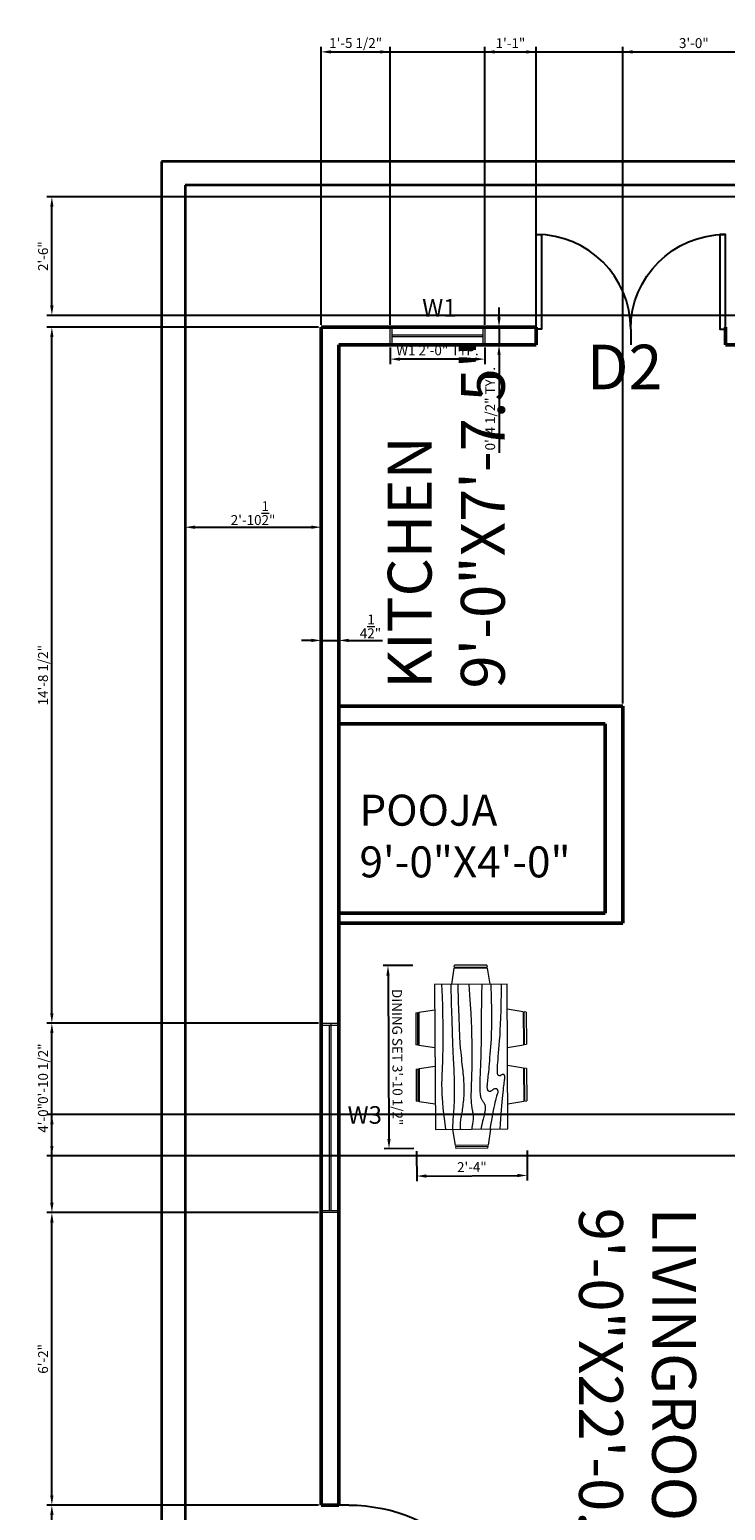
# Model space of a CAD drawing. Units: inches. Extents: x 2727 to 5054, y 1285 to 3233.
# Tile 2 of 3: x 2727 to 2903, y 1525 to 1900. Entities that reach past the tile are written whole.
import ezdxf

# ---------------------------------------------------------------- set-up
doc = ezdxf.new("R2010")
doc.units = ezdxf.units.IN
for name, color, linetype, lineweight in [('A-ANNO-TEXT', 1, 'Continuous', 18), ('A-AREA-IDEN', 1, 'Continuous', 18), ('A-WALL-SITE', 7, 'Continuous', 35), ('DIMENSIONS', 9, 'Continuous', 18), ('doors', 5, 'Continuous', 25), ('furniture', 8, 'Continuous', 18), ('walls', 7, 'Continuous', 50), ('windows', 3, 'Continuous', 18)]:
    doc.layers.add(name, color=color, linetype=linetype, lineweight=lineweight)
doc.styles.get("Standard").update_dxf_attribs({"font": 'arial.ttf'})
doc.dimstyles.new('ISO-25', dxfattribs={"dimtxt": 2.5, "dimasz": 2.5, "dimexe": 1.25, "dimexo": 0.625, "dimtad": 1, "dimlunit": 4, "dimtxsty": 'Standard', "dimcen": 2.5, "dimadec": 0, "dimazin": 0, "dimtfac": 1, "dimtmove": 0, "dimatfit": 3, "dimfxl": 1, "dimarcsym": 0})

# ---------------------------------------------------------------- blocks, each defined once
blk = doc.blocks.new('*U2')
for p, q in [((0, 0), (0, -5)), ((30, 0), (30, -5))]:
    blk.add_line(p, q)
blk.add_lwpolyline([(0, 0), (0, 30), (1.75, 30), (1.75, 0)], close=True)
blk.add_arc((0, 0), 30, 0, 90)
blk = doc.blocks.new('Dining Set - 36 x 72 in.')
for p, q in [((-22.2343, 26.00059), (-23.4847, 17.99762)), ((-22.2304, 26), (-5.7608, 26)), ((-22, 27.5), (-22.1562, 26.50042)), ((-5.8416, 26.5), (-22.1534, 26.5)), ((-22, 27.5), (-6, 27.5)), ((-5.8437, 26.49966), (-6, 27.5)), ((-4.5152, 17.99762), (-5.7655, 25.99926)), ((5.7657, 26.00059), (4.5153, 17.99762)), ((5.7696, 26), (22.2392, 26)), ((6, 27.5), (5.8438, 26.50042)), ((22.1584, 26.5), (5.8466, 26.5)), ((6, 27.5), (22, 27.5)), ((22.1563, 26.49966), (22, 27.5)), ((23.4848, 17.99762), (22.2345, 25.99926)), ((36, 18), (-36, 18)), ((-36, 18), (-36, -18)), ((36, -18), (36, 18)), ((-45.5, 8), (-44.5004, 8.15617)), ((-45.5, 8), (-45.5, -8)), ((-44.5, -8.15843), (-44.5, 8.15338)), ((-44.0006, 8.23428), (-35.9976, 9.48474)), ((-44, 8.23041), (-44, -8.23915)), ((44.0006, 8.23428), (35.9976, 9.48474)), ((44, 8.23041), (44, -8.23915)), ((44.5, -8.15843), (44.5, 8.15338)), ((45.5, 8), (44.5005, 8.15617)), ((45.5, 8), (45.5, -8)), ((-44.4997, -8.15631), (-45.5, -8)), ((-35.9976, -9.48476), (-43.9993, -8.2345)), ((35.9976, -9.48476), (43.9993, -8.2345)), ((44.4997, -8.15631), (45.5, -8)), ((-36, -18), (36, -18)), ((-22.2343, -26.0006), (-23.4847, -17.99762)), ((-4.5152, -17.99762), (-5.7655, -25.99928)), ((5.7657, -26.0006), (4.5153, -17.99762)), ((23.4848, -17.99762), (22.2345, -25.99928)), ((-22.2304, -26), (-5.7608, -26)), ((-22, -27.5), (-22.1562, -26.50044)), ((-5.8416, -26.5), (-22.1534, -26.5)), ((-22, -27.5), (-6, -27.5)), ((-5.8437, -26.49967), (-6, -27.5)), ((5.7696, -26), (22.2392, -26)), ((6, -27.5), (5.8438, -26.50044)), ((22.1584, -26.5), (5.8466, -26.5)), ((6, -27.5), (22, -27.5)), ((22.1563, -26.49967), (22, -27.5))]:
    blk.add_line(p, q)
for points in [[(-36, 15), (-31.1772, 14.97754), (-26.8079, 14.91406), (-22.8538, 14.81543), (-19.276, 14.6875), (-16.0362, 14.53613), (-13.0957, 14.36718), (-10.4159, 14.18652), (-7.9583, 14), (-5.6904, 13.81315), (-3.6035, 13.63021), (-1.6954, 13.45508), (0.0365, 13.29166), (1.5945, 13.14388), (2.9811, 13.01562), (4.1988, 12.9108), (5.25, 12.83333), (6.1393, 12.78613), (6.8802, 12.76823), (7.4883, 12.77767), (7.9792, 12.8125), (8.3685, 12.87077), (8.6719, 12.95052), (8.9049, 13.0498), (9.0833, 13.16666), (9.2205, 13.29899), (9.3216, 13.44401), (9.3895, 13.59879), (9.4271, 13.76041), (9.4373, 13.92594), (9.4232, 14.09245), (9.3875, 14.257), (9.3333, 14.41666), (9.2638, 14.56917), (9.1836, 14.71484), (9.0975, 14.85465), (9.0104, 14.98958), (8.9272, 15.1206), (8.8529, 15.2487), (8.7922, 15.37483), (8.75, 15.5), (8.7305, 15.62467), (8.7344, 15.74739), (8.7617, 15.86621), (8.8125, 15.97916), (8.8867, 16.08431), (8.9844, 16.17968), (9.1055, 16.26334), (9.25, 16.33333), (9.4189, 16.38802), (9.6172, 16.42708), (9.8506, 16.45052), (10.125, 16.45833), (10.4463, 16.45052), (10.8203, 16.42708), (11.2529, 16.38802), (11.75, 16.33333), (12.3184, 16.26318), (12.9694, 16.17838), (13.7151, 16.07991), (14.5677, 15.96875), (15.5395, 15.84586), (16.6426, 15.71224), (17.8893, 15.56884), (19.2917, 15.41666), (20.859, 15.25667), (22.5879, 15.08984), (24.4721, 14.91715), (26.5052, 14.73958), (28.6809, 14.5581), (30.9929, 14.3737), (33.4347, 14.18733), (36, 14)], [(-36, 10), (-28.9766, 10.14274), (-23.1725, 10.20442), (-18.4241, 10.19775), (-14.5677, 10.13541), (-11.4399, 10.03011), (-8.877, 9.89453), (-6.7154, 9.74137), (-4.7917, 9.58333), (-2.9698, 9.43082), (-1.2246, 9.28515), (0.4415, 9.14534), (2.026, 9.01041), (3.5266, 8.87939), (4.9408, 8.7513), (6.266, 8.62516), (7.5, 8.5), (8.6411, 8.37549), (9.6914, 8.2539), (10.6538, 8.13818), (11.5312, 8.03125), (12.3267, 7.93603), (13.043, 7.85547), (13.6831, 7.79248), (14.25, 7.75), (14.7471, 7.7303), (15.1797, 7.73307), (15.5537, 7.75732), (15.875, 7.80208), (16.1494, 7.86637), (16.3828, 7.94922), (16.5811, 8.04964), (16.75, 8.16666), (16.8944, 8.29915), (17.0143, 8.44531), (17.1089, 8.60319), (17.1771, 8.77083), (17.218, 8.94629), (17.2305, 9.1276), (17.2137, 9.31282), (17.1667, 9.5), (17.0895, 9.6875), (16.987, 9.875), (16.8649, 10.0625), (16.7292, 10.25), (16.5856, 10.4375), (16.4401, 10.625), (16.2985, 10.8125), (16.1667, 11), (16.05, 11.18733), (15.9518, 11.3737), (15.8752, 11.5581), (15.8229, 11.73958), (15.798, 11.91715), (15.8034, 12.08984), (15.842, 12.25667), (15.9167, 12.41666), (16.0295, 12.56836), (16.1784, 12.70833), (16.3605, 12.83268), (16.5729, 12.9375), (16.8127, 13.01888), (17.0768, 13.07291), (17.3625, 13.0957), (17.6667, 13.08333), (17.9894, 13.03312), (18.3418, 12.94726), (18.7382, 12.82918), (19.1927, 12.68229), (19.7195, 12.51001), (20.3327, 12.31575), (21.0465, 12.10294), (21.875, 11.875), (22.8357, 11.63354), (23.959, 11.37304), (25.2786, 11.08618), (26.8282, 10.76562), (28.6414, 10.40405), (30.752, 9.99414), (33.1936, 9.52856), (36, 9)], [(-36, 5.5), (-30.7157, 5.3348), (-26.069, 5.20963), (-21.9946, 5.11767), (-18.4271, 5.05208), (-15.3009, 5.00602), (-12.5508, 4.97265), (-10.1112, 4.94515), (-7.9167, 4.91666), (-5.909, 4.88167), (-4.0586, 4.83984), (-2.3429, 4.79215), (-0.7396, 4.73958), (0.7739, 4.6831), (2.22, 4.6237), (3.6213, 4.56233), (5, 4.5), (6.373, 4.43782), (7.7344, 4.3776), (9.0723, 4.32129), (10.375, 4.27083), (11.6309, 4.22819), (12.8281, 4.19531), (13.9551, 4.17415), (15, 4.16666), (15.954, 4.17448), (16.819, 4.19791), (17.6001, 4.23698), (18.3021, 4.29166), (18.9299, 4.36198), (19.4883, 4.44791), (19.9823, 4.54948), (20.4167, 4.66666), (20.7969, 4.79899), (21.1302, 4.94401), (21.4245, 5.09879), (21.6875, 5.26041), (21.9271, 5.42594), (22.1511, 5.59245), (22.3672, 5.757), (22.5834, 5.91666), (22.8065, 6.06868), (23.0404, 6.21093), (23.2879, 6.34147), (23.5521, 6.45833), (23.8358, 6.55957), (24.142, 6.64323), (24.4735, 6.70735), (24.8334, 6.75), (25.2235, 6.76969), (25.642, 6.76692), (26.0858, 6.74267), (26.5521, 6.69791), (27.0379, 6.63362), (27.5404, 6.55078), (28.0565, 6.45036), (28.5834, 6.33333), (29.1242, 6.19987), (29.7071, 6.04687), (30.3661, 5.87044), (31.1354, 5.66666), (32.0493, 5.43164), (33.142, 5.16146), (34.4475, 4.85221), (36, 4.5)], [(-36, -1), (-30.7915, -0.6591), (-26.0195, -0.38216), (-21.6519, -0.16284), (-17.6563, 0.00521), (-14.0005, 0.12833), (-10.6523, 0.21289), (-7.5796, 0.26522), (-4.75, 0.29166), (-2.134, 0.29793), (0.2878, 0.28711), (2.5317, 0.26163), (4.6146, 0.22396), (6.5529, 0.17651), (8.3633, 0.12174), (10.0623, 0.06209), (11.6667, 0), (13.1899, -0.06201), (14.6341, -0.1211), (15.9982, -0.17432), (17.2813, -0.21875), (18.4823, -0.25147), (19.6003, -0.26953), (20.6343, -0.27002), (21.5834, -0.25), (22.4481, -0.20768), (23.2357, -0.14584), (23.9549, -0.06836), (24.6146, 0.02083), (25.2235, 0.11784), (25.7904, 0.21875), (26.3241, 0.31966), (26.8334, 0.41666), (27.3265, 0.50618), (27.8099, 0.58593), (28.2894, 0.65397), (28.7709, 0.70833), (29.2601, 0.74707), (29.763, 0.76823), (30.2855, 0.76985), (30.8334, 0.75), (31.4088, 0.70784), (31.9994, 0.64713), (32.589, 0.57275), (33.1615, 0.48958), (33.7008, 0.4025), (34.1908, 0.3164), (34.6153, 0.23616), (34.9584, 0.16666), (35.2099, 0.11165), (35.3848, 0.07031), (35.504, 0.04069), (35.5886, 0.02083), (35.6594, 0.00879), (35.7377, 0.0026), (35.8442, 0.00032), (36, 0)], [(-36, -6.5), (-27.1843, -6.31267), (-20.084, -6.1263), (-14.469, -5.9419), (-10.1094, -5.76042), (-6.7752, -5.58285), (-4.2363, -5.41016), (-2.2629, -5.24333), (-0.625, -5.08334), (0.8708, -4.93099), (2.2715, -4.78646), (3.5872, -4.64974), (4.8281, -4.52084), (6.0046, -4.39974), (7.127, -4.28646), (8.2053, -4.18099), (9.25, -4.08334), (10.2705, -3.99382), (11.2734, -3.91407), (12.2647, -3.84603), (13.25, -3.79167), (14.2354, -3.75293), (15.2266, -3.73177), (16.2295, -3.73015), (17.25, -3.75), (18.2912, -3.79248), (19.3451, -3.85547), (20.4009, -3.93604), (21.4479, -4.03125), (22.4754, -4.13819), (23.4727, -4.25391), (24.4289, -4.37549), (25.3334, -4.5), (26.1785, -4.62492), (26.9694, -4.74935), (27.7145, -4.87281), (28.4219, -4.99479), (29.1, -5.11483), (29.7572, -5.23242), (30.4016, -5.34709), (31.0417, -5.45834), (31.6837, -5.56437), (32.3262, -5.65821), (32.9658, -5.73153), (33.599, -5.77604), (34.2224, -5.78345), (34.8327, -5.74545), (35.4264, -5.65373), (36, -5.5)], [(-36, -10), (-26.4022, -9.81299), (-18.4675, -9.62891), (-11.9839, -9.45069), (-6.7396, -9.28125), (-2.5226, -9.12354), (0.8789, -8.98047), (3.6769, -8.85498), (6.0833, -8.75), (8.2767, -8.66765), (10.3021, -8.60677), (12.1712, -8.56543), (13.8958, -8.54167), (15.4876, -8.53353), (16.9583, -8.53907), (18.3197, -8.55632), (19.5834, -8.58334), (20.7616, -8.61841), (21.8685, -8.66081), (22.9188, -8.71004), (23.9271, -8.76563), (24.9081, -8.82707), (25.8763, -8.89388), (26.8465, -8.96558), (27.8334, -9.04167), (28.8474, -9.12118), (29.8828, -9.20117), (30.93, -9.27824), (31.9792, -9.34896), (33.0205, -9.40991), (34.0443, -9.45768), (35.0407, -9.48885), (36, -9.5)], [(-36, -14.5), (-30.0881, -14.33513), (-25.0332, -14.21224), (-20.7312, -14.12647), (-17.0781, -14.07292), (-13.97, -14.04671), (-11.3027, -14.04297), (-8.9724, -14.05681), (-6.875, -14.08334), (-4.9224, -14.11833), (-3.0905, -14.16016), (-1.3709, -14.20785), (0.2448, -14.26042), (1.7647, -14.3169), (3.1973, -14.3763), (4.5507, -14.43767), (5.8333, -14.5), (7.0554, -14.5621), (8.235, -14.62175), (9.3922, -14.67652), (10.5469, -14.72396), (11.7192, -14.76164), (12.929, -14.78711), (14.1965, -14.79794), (15.5417, -14.79167), (16.9933, -14.76424), (18.6152, -14.70508), (20.4804, -14.60197), (22.6615, -14.44271), (25.2312, -14.21509), (28.2624, -13.9069), (31.8277, -13.50594), (36, -13)]]:
    blk.add_lwpolyline(points)
blk = doc.blocks.new('*D14')
at = {"layer": 'Defpoints', "color": 0, "transparency": 16777216}
for p in [(2766.39, 1793.24), (2800.89, 1793.24), (2800.89, 1773.7)]:
    blk.add_point(p, dxfattribs=at)
at = {"layer": 'DIMENSIONS', "color": 0, "lineweight": -2, "transparency": 16777216}
for p, q in [((2766.39, 1792.61), (2766.39, 1772.45)), ((2800.89, 1792.61), (2800.89, 1772.45)), ((2768.89, 1773.7), (2798.39, 1773.7))]:
    blk.add_line(p, q, dxfattribs=at)
at = {"layer": 'DIMENSIONS', "color": 0, "transparency": 16777216}
for points in [[(2768.89, 1774.12), (2768.89, 1773.28), (2766.39, 1773.7)], [(2798.39, 1774.12), (2798.39, 1773.28), (2800.89, 1773.7)]]:
    blk.add_solid(points, dxfattribs=at)
at = {"layer": 'DIMENSIONS', "color": 0, "transparency": 16777216, "insert": (2783.64, 1777.27), "char_height": 2.5, "attachment_point": 5}
blk.add_mtext('2\'-10{\\H1x;\\S1/2;}"', dxfattribs=at)
blk = doc.blocks.new('*D15')
at = {"layer": 'Defpoints', "color": 0, "transparency": 16777216}
for p in [(2800.89, 1749.45), (2805.39, 1749.45), (2805.39, 1745.01)]:
    blk.add_point(p, dxfattribs=at)
at = {"layer": 'DIMENSIONS', "color": 0, "lineweight": -2, "transparency": 16777216}
for p, q in [((2800.89, 1748.82), (2800.89, 1743.76)), ((2805.39, 1748.82), (2805.39, 1743.76)), ((2798.39, 1745.01), (2795.89, 1745.01)), ((2800.89, 1745.01), (2805.39, 1745.01)), ((2807.89, 1745.01), (2816.44, 1745.01))]:
    blk.add_line(p, q, dxfattribs=at)
at = {"layer": 'DIMENSIONS', "color": 0, "transparency": 16777216}
for points in [[(2798.39, 1745.43), (2798.39, 1744.6), (2800.89, 1745.01)], [(2807.89, 1745.43), (2807.89, 1744.6), (2805.39, 1745.01)]]:
    blk.add_solid(points, dxfattribs=at)
at = {"layer": 'DIMENSIONS', "color": 0, "transparency": 16777216, "insert": (2813.41, 1748.56), "char_height": 2.5, "attachment_point": 5}
blk.add_mtext('4{\\H1x;\\S1/2;}"', dxfattribs=at)
blk = doc.blocks.new('WIN-W1-24IN')
for p, q in [((0, 4.5), (24.02, 4.5)), ((0, 0), (0, 4.5)), ((0.5, 0), (0.5, 4.5)), ((23.52, 4.5), (23.52, 0)), ((24.02, 4.5), (24.02, 0)), ((24.02, 0), (0, 0)), ((0.5, 2.45), (23.52, 2.45)), ((0.5, 2.05), (23.52, 2.05))]:
    blk.add_line(p, q)
blk = doc.blocks.new('*D25')
at = {"layer": 'Defpoints', "color": 0, "transparency": 16777216}
for p in [(2818.38, 1819.89), (2818.38, 1816.29), (2842.4, 1819.89)]:
    blk.add_point(p, dxfattribs=at)
at = {"layer": 'DIMENSIONS', "color": 0, "lineweight": -2, "transparency": 16777216}
for p, q in [((2818.38, 1819.27), (2818.38, 1815.04)), ((2839.9, 1816.29), (2820.88, 1816.29)), ((2842.4, 1819.27), (2842.4, 1815.04))]:
    blk.add_line(p, q, dxfattribs=at)
at = {"layer": 'DIMENSIONS', "color": 0, "transparency": 16777216}
for points in [[(2820.88, 1816.7), (2820.88, 1815.87), (2818.38, 1816.29)], [(2839.9, 1816.7), (2839.9, 1815.87), (2842.4, 1816.29)]]:
    blk.add_solid(points, dxfattribs=at)
at = {"layer": 'DIMENSIONS', "color": 0, "transparency": 16777216, "insert": (2830.39, 1818.19), "char_height": 2.5, "attachment_point": 5}
blk.add_mtext('W1 2\'-0" TYP.', dxfattribs=at)
blk = doc.blocks.new('*D26')
at = {"layer": 'Defpoints', "color": 0, "transparency": 16777216}
for p in [(2842.4, 1824.39), (2842.4, 1819.89), (2846, 1819.89)]:
    blk.add_point(p, dxfattribs=at)
at = {"layer": 'DIMENSIONS', "color": 0, "lineweight": -2, "transparency": 16777216}
for p, q in [((2846, 1826.89), (2846, 1829.39)), ((2843.02, 1824.39), (2847.25, 1824.39)), ((2846, 1824.39), (2846, 1819.89)), ((2843.02, 1819.89), (2847.25, 1819.89)), ((2846, 1817.39), (2846, 1792.58))]:
    blk.add_line(p, q, dxfattribs=at)
at = {"layer": 'DIMENSIONS', "color": 0, "transparency": 16777216}
for points in [[(2845.58, 1826.89), (2846.42, 1826.89), (2846, 1824.39)], [(2845.58, 1817.39), (2846.42, 1817.39), (2846, 1819.89)]]:
    blk.add_solid(points, dxfattribs=at)
at = {"layer": 'DIMENSIONS', "color": 0, "transparency": 16777216, "insert": (2844.08, 1803.73), "char_height": 2.5, "attachment_point": 5, "rotation": 90}
blk.add_mtext('0\'-4 1/2" TYP.', dxfattribs=at)
blk = doc.blocks.new('*D37')
at = {"layer": 'Defpoints', "color": 0, "transparency": 16777216}
for p in [(2824.8, 1662.64), (2818.11, 1616.19), (2825.07, 1616.23)]:
    blk.add_point(p, dxfattribs=at)
at = {"layer": 'DIMENSIONS', "color": 0, "lineweight": -2, "transparency": 16777216}
for p, q in [((2824.17, 1662.63), (2816.59, 1662.59)), ((2817.85, 1660.09), (2818.09, 1618.69)), ((2824.44, 1616.22), (2816.86, 1616.18))]:
    blk.add_line(p, q, dxfattribs=at)
at = {"layer": 'DIMENSIONS', "color": 0, "transparency": 16777216}
for points in [[(2818.27, 1660.1), (2817.43, 1660.09), (2817.84, 1662.59)], [(2818.51, 1618.69), (2817.67, 1618.68), (2818.11, 1616.19)]]:
    blk.add_solid(points, dxfattribs=at)
at = {"layer": 'DIMENSIONS', "color": 0, "transparency": 16777216, "insert": (2819.89, 1639.4), "char_height": 2.5, "attachment_point": 5, "rotation": 270.3343}
blk.add_mtext('DINING SET 3\'-10 1/2"', dxfattribs=at)
blk = doc.blocks.new('*D38')
at = {"layer": 'Defpoints', "color": 0, "transparency": 16777216}
for p in [(2825.07, 1616.23), (2853.12, 1616.39), (2853.16, 1609.43)]:
    blk.add_point(p, dxfattribs=at)
at = {"layer": 'DIMENSIONS', "color": 0, "lineweight": -2, "transparency": 16777216}
for p, q in [((2825.07, 1615.6), (2825.12, 1608.02)), ((2853.12, 1615.77), (2853.16, 1608.18)), ((2827.61, 1609.28), (2850.66, 1609.41))]:
    blk.add_line(p, q, dxfattribs=at)
at = {"layer": 'DIMENSIONS', "color": 0, "transparency": 16777216}
for points in [[(2850.65, 1609.83), (2850.66, 1609), (2853.16, 1609.43)], [(2827.61, 1609.7), (2827.61, 1608.86), (2825.11, 1609.27)]]:
    blk.add_solid(points, dxfattribs=at)
at = {"layer": 'DIMENSIONS', "color": 0, "transparency": 16777216, "insert": (2839.12, 1611.23), "char_height": 2.5, "attachment_point": 5, "rotation": 0.3343}
blk.add_mtext('2\'-4"', dxfattribs=at)
blk = doc.blocks.new('*D41')
at = {"layer": 'Defpoints', "color": 0, "transparency": 16777216}
for p in [(3066.39, 1894.15), (3066.39, 1860.39), (2800.89, 1824.39)]:
    blk.add_point(p, dxfattribs=at)
at = {"layer": 'DIMENSIONS', "color": 0, "lineweight": -2, "transparency": 16777216}
for p, q in [((2800.89, 1825.02), (2800.89, 1895.4)), ((3066.39, 1861.02), (3066.39, 1895.4)), ((2803.39, 1894.15), (3063.89, 1894.15))]:
    blk.add_line(p, q, dxfattribs=at)
at = {"layer": 'DIMENSIONS', "color": 0, "transparency": 16777216}
for points in [[(2803.39, 1894.57), (2803.39, 1893.73), (2800.89, 1894.15)], [(3063.89, 1894.57), (3063.89, 1893.73), (3066.39, 1894.15)]]:
    blk.add_solid(points, dxfattribs=at)
at = {"layer": 'DIMENSIONS', "color": 0, "transparency": 16777216, "insert": (2933.64, 1896.07), "char_height": 2.5, "attachment_point": 5}
blk.add_mtext('22\'-1 1/2"', dxfattribs=at)
blk = doc.blocks.new('*D43')
at = {"layer": 'Defpoints', "color": 0, "transparency": 16777216}
for p in [(2732.63, 1525.89), (2800.89, 1525.89), (2800.89, 1483.89)]:
    blk.add_point(p, dxfattribs=at)
at = {"layer": 'DIMENSIONS', "color": 0, "lineweight": -2, "transparency": 16777216}
for p, q in [((2800.27, 1525.89), (2731.38, 1525.89)), ((2732.63, 1486.39), (2732.63, 1523.39)), ((2800.27, 1483.89), (2731.38, 1483.89))]:
    blk.add_line(p, q, dxfattribs=at)
at = {"layer": 'DIMENSIONS', "color": 0, "transparency": 16777216}
for points in [[(2732.21, 1523.39), (2733.05, 1523.39), (2732.63, 1525.89)], [(2732.21, 1486.39), (2733.05, 1486.39), (2732.63, 1483.89)]]:
    blk.add_solid(points, dxfattribs=at)
at = {"layer": 'DIMENSIONS', "color": 0, "transparency": 16777216, "insert": (2730.73, 1504.89), "char_height": 2.5, "attachment_point": 5, "rotation": 90}
blk.add_mtext('3\'-6"', dxfattribs=at)
blk = doc.blocks.new('*D45')
at = {"layer": 'Defpoints', "color": 0, "transparency": 16777216}
for p in [(2732.63, 1857.39), (2973.39, 1857.39), (2973.39, 1827.39)]:
    blk.add_point(p, dxfattribs=at)
at = {"layer": 'DIMENSIONS', "color": 0, "lineweight": -2, "transparency": 16777216}
for p, q in [((2972.77, 1857.39), (2731.38, 1857.39)), ((2732.63, 1829.89), (2732.63, 1854.89)), ((2972.77, 1827.39), (2731.38, 1827.39))]:
    blk.add_line(p, q, dxfattribs=at)
at = {"layer": 'DIMENSIONS', "color": 0, "transparency": 16777216}
for points in [[(2732.21, 1854.89), (2733.05, 1854.89), (2732.63, 1857.39)], [(2732.21, 1829.89), (2733.05, 1829.89), (2732.63, 1827.39)]]:
    blk.add_solid(points, dxfattribs=at)
at = {"layer": 'DIMENSIONS', "color": 0, "transparency": 16777216, "insert": (2730.73, 1842.39), "char_height": 2.5, "attachment_point": 5, "rotation": 90}
blk.add_mtext('2\'-6"', dxfattribs=at)
blk = doc.blocks.new('*D46')
at = {"layer": 'Defpoints', "color": 0, "transparency": 16777216}
for p in [(2732.63, 1648.01), (2800.89, 1648.01), (2800.89, 1600)]:
    blk.add_point(p, dxfattribs=at)
at = {"layer": 'DIMENSIONS', "color": 0, "lineweight": -2, "transparency": 16777216}
for p, q in [((2800.27, 1648.01), (2731.38, 1648.01)), ((2732.63, 1602.5), (2732.63, 1645.51)), ((2800.27, 1600), (2731.38, 1600))]:
    blk.add_line(p, q, dxfattribs=at)
at = {"layer": 'DIMENSIONS', "color": 0, "transparency": 16777216}
for points in [[(2732.21, 1645.51), (2733.05, 1645.51), (2732.63, 1648.01)], [(2732.21, 1602.5), (2733.05, 1602.5), (2732.63, 1600)]]:
    blk.add_solid(points, dxfattribs=at)
at = {"layer": 'DIMENSIONS', "color": 0, "transparency": 16777216, "insert": (2730.73, 1624.01), "char_height": 2.5, "attachment_point": 5, "rotation": 90}
blk.add_mtext('4\'-0"', dxfattribs=at)
blk = doc.blocks.new('*D48')
at = {"layer": 'Defpoints', "color": 0, "transparency": 16777216}
for p in [(2732.63, 1824.39), (2800.89, 1824.39), (2800.89, 1648.01)]:
    blk.add_point(p, dxfattribs=at)
at = {"layer": 'DIMENSIONS', "color": 0, "lineweight": -2, "transparency": 16777216}
for p, q in [((2800.27, 1824.39), (2731.38, 1824.39)), ((2732.63, 1650.51), (2732.63, 1821.89)), ((2800.27, 1648.01), (2731.38, 1648.01))]:
    blk.add_line(p, q, dxfattribs=at)
at = {"layer": 'DIMENSIONS', "color": 0, "transparency": 16777216}
for points in [[(2732.21, 1821.89), (2733.05, 1821.89), (2732.63, 1824.39)], [(2732.21, 1650.51), (2733.05, 1650.51), (2732.63, 1648.01)]]:
    blk.add_solid(points, dxfattribs=at)
at = {"layer": 'DIMENSIONS', "color": 0, "transparency": 16777216, "insert": (2730.71, 1736.2), "char_height": 2.5, "attachment_point": 5, "rotation": 90}
blk.add_mtext('14\'-8 1/2"', dxfattribs=at)
blk = doc.blocks.new('*D49')
at = {"layer": 'Defpoints', "color": 0, "transparency": 16777216}
for p in [(2732.63, 1600), (2800.89, 1600), (2800.89, 1525.89)]:
    blk.add_point(p, dxfattribs=at)
at = {"layer": 'DIMENSIONS', "color": 0, "lineweight": -2, "transparency": 16777216}
for p, q in [((2800.27, 1600), (2731.38, 1600)), ((2732.63, 1528.39), (2732.63, 1597.5)), ((2800.27, 1525.89), (2731.38, 1525.89))]:
    blk.add_line(p, q, dxfattribs=at)
at = {"layer": 'DIMENSIONS', "color": 0, "transparency": 16777216}
for points in [[(2732.21, 1597.5), (2733.05, 1597.5), (2732.63, 1600)], [(2732.21, 1528.39), (2733.05, 1528.39), (2732.63, 1525.89)]]:
    blk.add_solid(points, dxfattribs=at)
at = {"layer": 'DIMENSIONS', "color": 0, "transparency": 16777216, "insert": (2730.73, 1562.94), "char_height": 2.5, "attachment_point": 5, "rotation": 90}
blk.add_mtext('6\'-2"', dxfattribs=at)
blk = doc.blocks.new('*D54')
at = {"layer": 'Defpoints', "color": 0, "transparency": 16777216}
for p in [(2818.38, 1894.15), (2800.89, 1824.39), (2818.38, 1824.39)]:
    blk.add_point(p, dxfattribs=at)
at = {"layer": 'DIMENSIONS', "color": 0, "lineweight": -2, "transparency": 16777216}
for p, q in [((2800.89, 1825.02), (2800.89, 1895.4)), ((2818.38, 1825.02), (2818.38, 1895.4)), ((2803.39, 1894.15), (2815.88, 1894.15))]:
    blk.add_line(p, q, dxfattribs=at)
at = {"layer": 'DIMENSIONS', "color": 0, "transparency": 16777216}
for points in [[(2803.39, 1894.57), (2803.39, 1893.73), (2800.89, 1894.15)], [(2815.88, 1894.57), (2815.88, 1893.73), (2818.38, 1894.15)]]:
    blk.add_solid(points, dxfattribs=at)
at = {"layer": 'DIMENSIONS', "color": 0, "transparency": 16777216, "insert": (2809.64, 1896.07), "char_height": 2.5, "attachment_point": 5}
blk.add_mtext('1\'-5 1/2"', dxfattribs=at)
blk = doc.blocks.new('*D55')
at = {"layer": 'Defpoints', "color": 0, "transparency": 16777216}
for p in [(2855.39, 1894.15), (2842.4, 1824.39), (2855.39, 1824.39)]:
    blk.add_point(p, dxfattribs=at)
at = {"layer": 'DIMENSIONS', "color": 0, "lineweight": -2, "transparency": 16777216}
for p, q in [((2842.4, 1825.02), (2842.4, 1895.4)), ((2855.39, 1825.02), (2855.39, 1895.4)), ((2844.9, 1894.15), (2852.89, 1894.15))]:
    blk.add_line(p, q, dxfattribs=at)
at = {"layer": 'DIMENSIONS', "color": 0, "transparency": 16777216}
for points in [[(2844.9, 1894.57), (2844.9, 1893.73), (2842.4, 1894.15)], [(2852.89, 1894.57), (2852.89, 1893.73), (2855.39, 1894.15)]]:
    blk.add_solid(points, dxfattribs=at)
at = {"layer": 'DIMENSIONS', "color": 0, "transparency": 16777216, "insert": (2848.89, 1896.03), "char_height": 2.5, "attachment_point": 5}
blk.add_mtext('1\'-1"', dxfattribs=at)
blk = doc.blocks.new('*D56')
at = {"layer": 'Defpoints', "color": 0, "transparency": 16777216}
for p in [(2913.39, 1894.15), (2877.39, 1728.39), (2913.39, 1723.89)]:
    blk.add_point(p, dxfattribs=at)
at = {"layer": 'DIMENSIONS', "color": 0, "lineweight": -2, "transparency": 16777216}
for p, q in [((2877.39, 1729.02), (2877.39, 1895.4)), ((2913.39, 1724.52), (2913.39, 1895.4)), ((2879.89, 1894.15), (2910.89, 1894.15))]:
    blk.add_line(p, q, dxfattribs=at)
at = {"layer": 'DIMENSIONS', "color": 0, "transparency": 16777216}
for points in [[(2879.89, 1894.57), (2879.89, 1893.73), (2877.39, 1894.15)], [(2910.89, 1894.57), (2910.89, 1893.73), (2913.39, 1894.15)]]:
    blk.add_solid(points, dxfattribs=at)
at = {"layer": 'DIMENSIONS', "color": 0, "transparency": 16777216, "insert": (2895.39, 1896.05), "char_height": 2.5, "attachment_point": 5}
blk.add_mtext('3\'-0"', dxfattribs=at)
blk = doc.blocks.new('*D58')
at = {"layer": 'Defpoints', "color": 0, "transparency": 16777216}
for p in [(2732.63, 1624.89), (3061.89, 1624.89), (3061.89, 1614.39)]:
    blk.add_point(p, dxfattribs=at)
at = {"layer": 'DIMENSIONS', "color": 0, "lineweight": -2, "transparency": 16777216}
for p, q in [((2732.63, 1624.89), (2732.63, 1643.05)), ((3061.27, 1624.89), (2731.38, 1624.89)), ((2732.63, 1616.89), (2732.63, 1622.39)), ((3061.27, 1614.39), (2731.38, 1614.39))]:
    blk.add_line(p, q, dxfattribs=at)
at = {"layer": 'DIMENSIONS', "color": 0, "transparency": 16777216}
for points in [[(2732.21, 1622.39), (2733.05, 1622.39), (2732.63, 1624.89)], [(2732.21, 1616.89), (2733.05, 1616.89), (2732.63, 1614.39)]]:
    blk.add_solid(points, dxfattribs=at)
at = {"layer": 'DIMENSIONS', "color": 0, "transparency": 16777216, "insert": (2730.71, 1635.22), "char_height": 2.5, "attachment_point": 5, "rotation": 90}
blk.add_mtext('0\'-10 1/2"', dxfattribs=at)

msp = doc.modelspace()

# ---------------------------------------------------------------- linework, layer by layer
at = {"layer": 'A-WALL-SITE'}
for p, q in [((3084.39, 1866.39), (2760.39, 1866.39)), ((2760.39, 1866.39), (2760.39, 1314.39)), ((2766.39, 1860.39), (2766.39, 1320.39)), ((3078.39, 1860.39), (2766.39, 1860.39))]:
    msp.add_line(p, q, dxfattribs=at)
at = {"layer": 'walls'}
for p, q in [((2800.89, 1525.89), (2800.89, 1824.39)), ((2855.39, 1824.39), (2800.89, 1824.39)), ((2855.39, 1824.39), (2853.39, 1824.39)), ((2855.39, 1824.39), (2855.39, 1819.89)), ((2903.39, 1819.89), (2903.39, 1824.39)), ((2805.39, 1525.89), (2805.39, 1819.89)), ((2855.39, 1819.89), (2805.39, 1819.89)), ((3061.89, 1819.89), (2903.39, 1819.89)), ((2877.39, 1728.39), (2805.39, 1728.39)), ((2877.39, 1673.39), (2877.39, 1728.39)), ((2872.89, 1723.89), (2805.39, 1723.89)), ((2872.89, 1675.89), (2872.89, 1723.89)), ((2872.89, 1675.89), (2805.39, 1675.89)), ((2805.39, 1673.39), (2877.39, 1673.39)), ((2877.39, 1673.39), (2805.39, 1673.39)), ((2800.89, 1525.89), (2805.39, 1525.89))]:
    msp.add_line(p, q, dxfattribs=at)
at = {"layer": 'windows'}
for p, q in [((2800.89, 1599.998), (2800.89, 1648.014)), ((2800.89, 1648.014), (2805.39, 1648.014)), ((2800.89, 1647.514), (2805.39, 1647.514)), ((2802.94, 1647.514), (2802.94, 1600.498)), ((2803.34, 1648.014), (2803.34, 1600.498)), ((2805.39, 1648.014), (2805.39, 1599.998)), ((2805.39, 1600.498), (2800.89, 1600.498)), ((2805.39, 1599.998), (2800.89, 1599.998))]:
    msp.add_line(p, q, dxfattribs=at)

# ---------------------------------------------------------------- block references
at = {"layer": 'doors', "yscale": 0.8, "zscale": 0.8}
for p, xscale in [((2855.39, 1823.89), 0.8), ((2903.39, 1823.89), -0.8)]:
    msp.add_blockref('*U2', p, dxfattribs=dict(at, xscale=xscale))
at = {"layer": 'doors', "xscale": -1.399999999999999, "yscale": 1.399999999999999, "zscale": 1.399999999999999, "rotation": 270}
msp.add_blockref('*U2', (2807.89, 1483.89), dxfattribs=at)
at = {"layer": 'furniture', "xscale": 0.5099935498076289, "yscale": 0.5099935498076289, "zscale": 0.5099935498076289, "rotation": 270.3343210164401}
msp.add_blockref('Dining Set - 36 x 72 in.', (2838.957, 1639.513), dxfattribs=at)
at = {"layer": 'windows', "rotation": 180}
msp.add_blockref('WIN-W1-24IN', (2842.398, 1824.39), dxfattribs=at)

# ---------------------------------------------------------------- texts
at = {"layer": 'A-ANNO-TEXT', "char_height": 4.4548, "attachment_point": 1}
for s, insert in [('W1', (2826.514, 1831.529)), ('W3', (2807.602, 1626.984))]:
    msp.add_mtext_dynamic_manual_height_columns(s, width=0.75599, gutter_width=22.274, heights=[0], dxfattribs=dict(at, insert=insert))
at = {"layer": 'A-ANNO-TEXT', "insert": (2868.225, 1819.955), "char_height": 11.3069, "attachment_point": 1}
msp.add_mtext('D2', dxfattribs=at)
at = {"layer": 'A-AREA-IDEN', "char_height": 11.11906, "attachment_point": 1}
for s, insert, rotation in [('KITCHEN\\P9\'-0"X7\'-7.5"', (2817.795, 1732.81), 90), ('LIVINGROOM\\P9\'-0"X22\'-0.5"', (2895.951, 1601.252), 270)]:
    msp.add_mtext_dynamic_manual_height_columns(s, width=20.03048, gutter_width=55.595, heights=[0], dxfattribs=dict(at, insert=insert, rotation=rotation))
at = {"layer": 'A-AREA-IDEN', "insert": (2810.623, 1705.921), "char_height": 7.8579, "attachment_point": 1}
msp.add_mtext_dynamic_manual_height_columns('POOJA\\P9\'-0"X4\'-0"', width=0.81491, gutter_width=39.289, heights=[0], dxfattribs=at)

# ---------------------------------------------------------------- dimensions: what is measured, and where the dimension line sits
at = {"layer": 'DIMENSIONS'}
for base, p1, p2, override, picture, middle in [((3066.39, 1894.15), (2800.89, 1824.39), (3066.39, 1860.39), {"dimdec": 1, "dimlfac": 1, "dimrnd": 0, "dimzin": 1, "dimdsep": 46, "dimlunit": 4, "dimfrac": 2}, '*D41', (2933.64, 1896.068)), ((2818.382, 1894.15), (2800.89, 1824.39), (2818.382, 1824.39), {"dimdec": 1, "dimlfac": 1, "dimrnd": 0, "dimzin": 1, "dimdsep": 46, "dimlunit": 4, "dimfrac": 2}, '*D54', (2809.636, 1896.068)), ((2855.39, 1894.15), (2842.398, 1824.39), (2855.39, 1824.39), {"dimdec": 1, "dimlfac": 1, "dimrnd": 0, "dimzin": 1, "dimdsep": 46, "dimlunit": 4, "dimfrac": 2}, '*D55', (2848.894, 1896.03)), ((2913.39, 1894.15), (2877.39, 1728.39), (2913.39, 1723.89), {"dimdec": 1, "dimlfac": 1, "dimrnd": 0, "dimzin": 1, "dimdsep": 46, "dimlunit": 4, "dimfrac": 2}, '*D56', (2895.39, 1896.052)), ((2800.89, 1773.7), (2766.39, 1793.239), (2800.89, 1793.239), {"dimclrd": 0, "dimclre": 0, "dimclrt": 0}, '*D14', (2783.64, 1777.273)), ((2805.39, 1745.013), (2800.89, 1749.449), (2805.39, 1749.449), {"dimclrd": 0, "dimclre": 0, "dimclrt": 0}, '*D15', (2813.414, 1748.565))]:
    dim = msp.add_linear_dim(base=base, p1=p1, p2=p2, dimstyle='ISO-25', override=override, dxfattribs=at)
    dim.commit()
    dim.dimension.update_dxf_attribs({"geometry": picture, "text_midpoint": middle})
for base, p1, p2, angle, picture, middle in [((2732.63, 1857.39), (2973.39, 1827.39), (2973.39, 1857.39), 90, '*D45', (2730.729, 1842.39)), ((2732.63, 1824.39), (2800.89, 1648.014), (2800.89, 1824.39), 90, '*D48', (2730.713, 1736.202)), ((2732.63, 1648.014), (2800.89, 1599.998), (2800.89, 1648.014), 90, '*D46', (2730.729, 1624.006)), ((2732.63, 1624.89), (3061.89, 1614.39), (3061.89, 1624.89), 90, '*D58', (2730.713, 1635.222)), ((2853.157, 1609.429), (2825.067, 1616.227), (2853.116, 1616.39), 0.33432, '*D38', (2839.122, 1611.227)), ((2732.63, 1599.998), (2800.89, 1525.89), (2800.89, 1599.998), 90, '*D49', (2730.729, 1562.944)), ((2732.63, 1525.89), (2800.89, 1483.89), (2800.89, 1525.89), 90, '*D43', (2730.728, 1504.89))]:
    dim = msp.add_linear_dim(base=base, p1=p1, p2=p2, angle=angle, dimstyle='ISO-25', override={"dimdec": 1, "dimlfac": 1, "dimrnd": 0, "dimzin": 1, "dimdsep": 46, "dimlunit": 4, "dimfrac": 2}, dxfattribs=at)
    dim.commit()
    dim.dimension.update_dxf_attribs({"geometry": picture, "text_midpoint": middle})
for base, p1, p2, angle, text, picture, middle in [((2846.001, 1819.89), (2842.398, 1824.39), (2842.398, 1819.89), 270, '<> TYP.', '*D26', (2844.083, 1803.733)), ((2818.382, 1816.288), (2842.398, 1819.89), (2818.382, 1819.89), 180, 'W1 <> TYP.', '*D25', (2830.39, 1818.189)), ((2818.106, 1616.186), (2824.797, 1662.635), (2825.067, 1616.227), 270.33432, 'DINING SET <>', '*D37', (2819.889, 1639.401))]:
    dim = msp.add_linear_dim(base=base, p1=p1, p2=p2, angle=angle, text=text, dimstyle='ISO-25', override={"dimdec": 1, "dimlfac": 1, "dimrnd": 0, "dimzin": 1, "dimdsep": 46, "dimlunit": 4, "dimfrac": 2}, dxfattribs=at)
    dim.commit()
    dim.dimension.update_dxf_attribs({"geometry": picture, "text_midpoint": middle})

doc.saveas('drawing.dxf')
